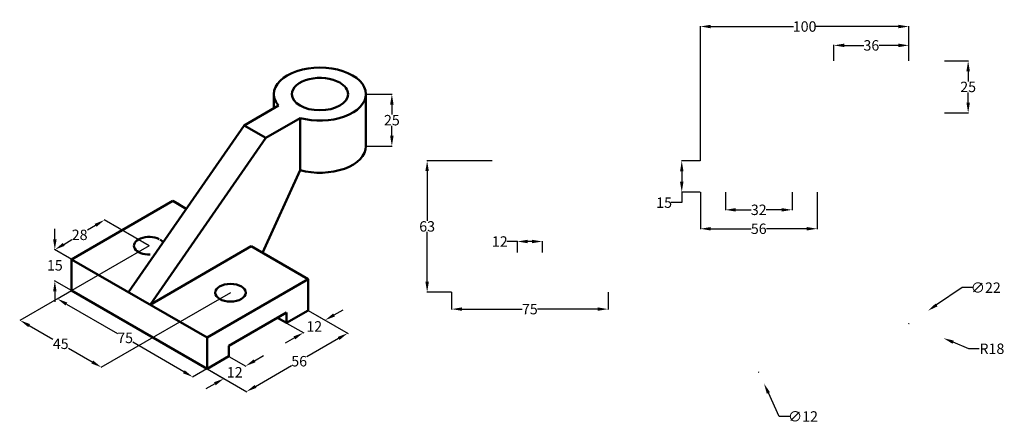
# Model space of a CAD drawing. Units: millimetres. Extents: x -452 to 20, y -1277 to -1083.
import ezdxf

# ---------------------------------------------------------------- set-up
doc = ezdxf.new("R2010")
doc.units = ezdxf.units.MM
doc.layers.add('M-DIMS', color=2, linetype='Continuous', lineweight=25)
doc.layers.add('M-OUTL', color=7, linetype='Continuous', lineweight=50)
doc.styles.get("Standard").update_dxf_attribs({"font": 'arial.ttf'})
doc.dimstyles.get("Standard").update_dxf_attribs({"dimtxt": 5, "dimasz": 5, "dimexe": 0.18, "dimexo": 0.0625, "dimgap": 0.09, "dimtad": 0, "dimtih": 1, "dimtoh": 1, "dimdec": 0, "dimzin": 0, "dimdsep": 46, "dimtxsty": 'Standard', "dimcen": 0.09, "dimadec": 0, "dimazin": 0, "dimtfac": 1, "dimtdec": 0, "dimtofl": 0, "dimtmove": 0, "dimatfit": 3, "dimfxl": 1, "dimtolj": 1, "dimtzin": 0, "dimarcsym": 0})

# ---------------------------------------------------------------- blocks, each defined once
blk = doc.blocks.new('*D1')
at = {"layer": 'Defpoints', "color": 0, "transparency": 16777216}
for p in [(-427.19, -1197.94), (-435.2, -1208.32), (-427.19, -1212.94)]:
    blk.add_point(p, dxfattribs=at)
at = {"layer": 'M-DIMS', "color": 0, "lineweight": -2, "transparency": 16777216}
for p, q in [((-435.2, -1188.32), (-435.2, -1183.32)), ((-427.25, -1197.9), (-435.38, -1193.21)), ((-427.25, -1212.9), (-435.38, -1208.21)), ((-435.2, -1213.32), (-435.2, -1218.32))]:
    blk.add_line(p, q, dxfattribs=at)
at = {"layer": 'M-DIMS', "color": 0, "transparency": 16777216}
for points in [[(-436.03, -1188.32), (-434.36, -1188.32), (-435.2, -1193.32)], [(-436.03, -1213.32), (-434.36, -1213.32), (-435.2, -1208.32)]]:
    blk.add_solid(points, dxfattribs=at)
at = {"layer": 'M-DIMS', "color": 0, "transparency": 16777216, "insert": (-435.2, -1200.82), "char_height": 5, "attachment_point": 5}
blk.add_mtext('\\A1;15', dxfattribs=at)
blk = doc.blocks.new('*D2')
at = {"layer": 'Defpoints', "color": 0, "transparency": 16777216}
for p in [(-427.19, -1212.94), (-362.24, -1250.44), (-369.03, -1254.36)]:
    blk.add_point(p, dxfattribs=at)
at = {"layer": 'M-DIMS', "color": 0, "lineweight": -2, "transparency": 16777216}
for p, q in [((-427.25, -1212.97), (-434.16, -1216.96)), ((-429.65, -1219.36), (-405.17, -1233.49)), ((-373.36, -1251.86), (-397.84, -1237.73)), ((-362.3, -1250.47), (-369.21, -1254.46))]:
    blk.add_line(p, q, dxfattribs=at)
at = {"layer": 'M-DIMS', "color": 0, "transparency": 16777216}
for points in [[(-429.23, -1218.64), (-430.07, -1220.08), (-433.98, -1216.86)], [(-372.94, -1251.14), (-373.78, -1252.58), (-369.03, -1254.36)]]:
    blk.add_solid(points, dxfattribs=at)
at = {"layer": 'M-DIMS', "color": 0, "transparency": 16777216, "insert": (-401.51, -1235.61), "char_height": 5, "attachment_point": 5}
blk.add_mtext('\\A1;75', dxfattribs=at)
blk = doc.blocks.new('*D3')
at = {"layer": 'Defpoints', "color": 0, "transparency": 16777216}
for p in [(-313.74, -1222.44), (-294.8, -1233.37), (-362.24, -1250.44)]:
    blk.add_point(p, dxfattribs=at)
at = {"layer": 'M-DIMS', "color": 0, "lineweight": -2, "transparency": 16777216}
for p, q in [((-313.68, -1222.47), (-294.62, -1233.48)), ((-299.13, -1235.87), (-314.38, -1244.68)), ((-362.17, -1250.47), (-343.12, -1261.48)), ((-338.97, -1258.87), (-321.72, -1248.91))]:
    blk.add_line(p, q, dxfattribs=at)
at = {"layer": 'M-DIMS', "color": 0, "transparency": 16777216}
for points in [[(-299.55, -1235.15), (-298.72, -1236.59), (-294.8, -1233.37)], [(-339.39, -1258.15), (-338.55, -1259.59), (-343.3, -1261.37)]]:
    blk.add_solid(points, dxfattribs=at)
at = {"layer": 'M-DIMS', "color": 0, "transparency": 16777216, "insert": (-318.05, -1246.79), "char_height": 5, "attachment_point": 5}
blk.add_mtext('\\A1;56', dxfattribs=at)
blk = doc.blocks.new('*D4')
at = {"layer": 'Defpoints', "color": 0, "transparency": 16777216}
for p in [(-313.74, -1222.44), (-305.64, -1227.11), (-324.13, -1228.44)]:
    blk.add_point(p, dxfattribs=at)
at = {"layer": 'M-DIMS', "color": 0, "lineweight": -2, "transparency": 16777216}
for p, q in [((-313.68, -1222.47), (-305.46, -1227.22)), ((-301.31, -1224.61), (-296.98, -1222.11)), ((-324.07, -1228.47), (-315.86, -1233.22)), ((-320.37, -1235.61), (-324.7, -1238.11))]:
    blk.add_line(p, q, dxfattribs=at)
at = {"layer": 'M-DIMS', "color": 0, "transparency": 16777216}
for points in [[(-301.73, -1223.89), (-300.9, -1225.33), (-305.64, -1227.11)], [(-320.78, -1234.89), (-319.95, -1236.33), (-316.04, -1233.11)]]:
    blk.add_solid(points, dxfattribs=at)
at = {"layer": 'M-DIMS', "color": 0, "transparency": 16777216, "insert": (-310.84, -1230.11), "char_height": 5, "attachment_point": 5}
blk.add_mtext('\\A1;12', dxfattribs=at)
blk = doc.blocks.new('*D5')
at = {"layer": 'Defpoints', "color": 0, "transparency": 16777216}
for p in [(-351.85, -1244.44), (-362.24, -1250.44), (-343.75, -1249.11)]:
    blk.add_point(p, dxfattribs=at)
at = {"layer": 'M-DIMS', "color": 0, "lineweight": -2, "transparency": 16777216}
for p, q in [((-351.78, -1244.47), (-343.57, -1249.22)), ((-339.42, -1246.61), (-335.09, -1244.11)), ((-362.17, -1250.47), (-353.96, -1255.22)), ((-358.47, -1257.61), (-362.8, -1260.11))]:
    blk.add_line(p, q, dxfattribs=at)
at = {"layer": 'M-DIMS', "color": 0, "transparency": 16777216}
for points in [[(-339.84, -1245.89), (-339, -1247.33), (-343.75, -1249.11)], [(-358.89, -1256.89), (-358.06, -1258.33), (-354.14, -1255.11)]]:
    blk.add_solid(points, dxfattribs=at)
at = {"layer": 'M-DIMS', "color": 0, "transparency": 16777216, "insert": (-348.95, -1252.11), "char_height": 5, "attachment_point": 5}
blk.add_mtext('\\A1;12', dxfattribs=at)
blk = doc.blocks.new('*D6')
at = {"layer": 'Defpoints', "color": 0, "transparency": 16777216}
for p in [(-435.2, -1193.32), (-389.95, -1191.44), (-413.75, -1205.7)]:
    blk.add_point(p, dxfattribs=at)
at = {"layer": 'M-DIMS', "color": 0, "lineweight": -2, "transparency": 16777216}
for p, q in [((-390.01, -1191.4), (-411.57, -1178.95)), ((-415.68, -1181.63), (-419.58, -1183.96)), ((-430.91, -1190.75), (-427.01, -1188.41)), ((-413.81, -1205.66), (-435.38, -1193.21))]:
    blk.add_line(p, q, dxfattribs=at)
at = {"layer": 'M-DIMS', "color": 0, "transparency": 16777216}
for points in [[(-416.11, -1180.91), (-415.26, -1182.34), (-411.39, -1179.06)], [(-431.34, -1190.03), (-430.48, -1191.46), (-435.2, -1193.32)]]:
    blk.add_solid(points, dxfattribs=at)
at = {"layer": 'M-DIMS', "color": 0, "transparency": 16777216, "insert": (-423.3, -1186.19), "char_height": 5, "attachment_point": 5}
blk.add_mtext('\\A1;28', dxfattribs=at)
blk = doc.blocks.new('*D7')
at = {"layer": 'Defpoints', "color": 0, "transparency": 16777216}
for p in [(-389.95, -1191.44), (-350.98, -1213.94), (-412.9, -1249.69)]:
    blk.add_point(p, dxfattribs=at)
at = {"layer": 'M-DIMS', "color": 0, "lineweight": -2, "transparency": 16777216}
for p, q in [((-390.01, -1191.47), (-452.05, -1227.29)), ((-351.04, -1213.97), (-413.08, -1249.79)), ((-447.54, -1229.69), (-436.18, -1236.25)), ((-417.23, -1247.19), (-428.6, -1240.63))]:
    blk.add_line(p, q, dxfattribs=at)
at = {"layer": 'M-DIMS', "color": 0, "transparency": 16777216}
for points in [[(-447.13, -1228.97), (-447.96, -1230.41), (-451.87, -1227.19)], [(-416.82, -1246.47), (-417.65, -1247.91), (-412.9, -1249.69)]]:
    blk.add_solid(points, dxfattribs=at)
at = {"layer": 'M-DIMS', "color": 0, "transparency": 16777216, "insert": (-432.39, -1238.44), "char_height": 5, "attachment_point": 5}
blk.add_mtext('\\A1;45', dxfattribs=at)
blk = doc.blocks.new('*D8')
at = {"layer": 'Defpoints', "color": 0, "transparency": 16777216}
for p in [(-244.95, -1213.64), (-169.95, -1213.64), (-244.95, -1221.81)]:
    blk.add_point(p, dxfattribs=at)
at = {"layer": 'M-DIMS', "color": 0, "lineweight": -2, "transparency": 16777216}
for p, q in [((-244.95, -1213.71), (-244.95, -1221.99)), ((-169.95, -1213.71), (-169.95, -1221.99)), ((-239.95, -1221.81), (-211.12, -1221.81)), ((-174.95, -1221.81), (-203.78, -1221.81))]:
    blk.add_line(p, q, dxfattribs=at)
at = {"layer": 'M-DIMS', "color": 0, "transparency": 16777216}
for points in [[(-239.95, -1220.98), (-239.95, -1222.64), (-244.95, -1221.81)], [(-174.95, -1220.98), (-174.95, -1222.64), (-169.95, -1221.81)]]:
    blk.add_solid(points, dxfattribs=at)
at = {"layer": 'M-DIMS', "color": 0, "transparency": 16777216, "insert": (-207.45, -1221.81), "char_height": 5, "attachment_point": 5}
blk.add_mtext('\\A1;75', dxfattribs=at)
blk = doc.blocks.new('*D9')
at = {"layer": 'Defpoints', "color": 0, "transparency": 16777216}
for p in [(-125.71, -1150.74), (-134.62, -1165.74), (-125.71, -1165.74)]:
    blk.add_point(p, dxfattribs=at)
at = {"layer": 'M-DIMS', "color": 0, "lineweight": -2, "transparency": 16777216}
for p, q in [((-125.78, -1150.74), (-134.8, -1150.74)), ((-134.62, -1155.74), (-134.62, -1160.74)), ((-125.78, -1165.74), (-134.8, -1165.74)), ((-134.62, -1165.74), (-134.62, -1170.74)), ((-134.62, -1170.74), (-139.62, -1170.74))]:
    blk.add_line(p, q, dxfattribs=at)
at = {"layer": 'M-DIMS', "color": 0, "transparency": 16777216}
for points in [[(-135.45, -1155.74), (-133.78, -1155.74), (-134.62, -1150.74)], [(-135.45, -1160.74), (-133.78, -1160.74), (-134.62, -1165.74)]]:
    blk.add_solid(points, dxfattribs=at)
at = {"layer": 'M-DIMS', "color": 0, "transparency": 16777216, "insert": (-143.07, -1170.74), "char_height": 5, "attachment_point": 5}
blk.add_mtext('\\A1;15', dxfattribs=at)
blk = doc.blocks.new('*D10')
at = {"layer": 'Defpoints', "color": 0, "transparency": 16777216}
for p in [(-113.71, -1165.74), (-81.71, -1165.74), (-81.71, -1174.19)]:
    blk.add_point(p, dxfattribs=at)
at = {"layer": 'M-DIMS', "color": 0, "lineweight": -2, "transparency": 16777216}
for p, q in [((-113.71, -1165.8), (-113.71, -1174.37)), ((-81.71, -1165.8), (-81.71, -1174.37)), ((-108.71, -1174.19), (-101.36, -1174.19)), ((-86.71, -1174.19), (-94.07, -1174.19))]:
    blk.add_line(p, q, dxfattribs=at)
at = {"layer": 'M-DIMS', "color": 0, "transparency": 16777216}
for points in [[(-108.71, -1173.36), (-108.71, -1175.02), (-113.71, -1174.19)], [(-86.71, -1173.36), (-86.71, -1175.02), (-81.71, -1174.19)]]:
    blk.add_solid(points, dxfattribs=at)
at = {"layer": 'M-DIMS', "color": 0, "transparency": 16777216, "insert": (-97.71, -1174.19), "char_height": 5, "attachment_point": 5}
blk.add_mtext('\\A1;32', dxfattribs=at)
blk = doc.blocks.new('*D11')
at = {"layer": 'Defpoints', "color": 0, "transparency": 16777216}
for p in [(-125.71, -1165.74), (-69.71, -1165.74), (-69.71, -1183.27)]:
    blk.add_point(p, dxfattribs=at)
at = {"layer": 'M-DIMS', "color": 0, "lineweight": -2, "transparency": 16777216}
for p, q in [((-125.71, -1165.8), (-125.71, -1183.45)), ((-69.71, -1165.8), (-69.71, -1183.45)), ((-120.71, -1183.27), (-101.38, -1183.27)), ((-74.71, -1183.27), (-94.04, -1183.27))]:
    blk.add_line(p, q, dxfattribs=at)
at = {"layer": 'M-DIMS', "color": 0, "transparency": 16777216}
for points in [[(-120.71, -1182.44), (-120.71, -1184.11), (-125.71, -1183.27)], [(-74.71, -1182.44), (-74.71, -1184.11), (-69.71, -1183.27)]]:
    blk.add_solid(points, dxfattribs=at)
at = {"layer": 'M-DIMS', "color": 0, "transparency": 16777216, "insert": (-97.71, -1183.27), "char_height": 5, "attachment_point": 5}
blk.add_mtext('\\A1;56', dxfattribs=at)
blk = doc.blocks.new('*D12')
at = {"layer": 'Defpoints', "color": 0, "transparency": 16777216}
for p in [(-8.71, -1102.74), (2.7, -1102.74), (-8.71, -1127.74)]:
    blk.add_point(p, dxfattribs=at)
at = {"layer": 'M-DIMS', "color": 0, "lineweight": -2, "transparency": 16777216}
for p, q in [((-8.65, -1102.74), (2.88, -1102.74)), ((2.7, -1107.74), (2.7, -1112.6)), ((2.7, -1122.74), (2.7, -1117.88)), ((-8.65, -1127.74), (2.88, -1127.74))]:
    blk.add_line(p, q, dxfattribs=at)
at = {"layer": 'M-DIMS', "color": 0, "transparency": 16777216}
for points in [[(1.86, -1107.74), (3.53, -1107.74), (2.7, -1102.74)], [(1.86, -1122.74), (3.53, -1122.74), (2.7, -1127.74)]]:
    blk.add_solid(points, dxfattribs=at)
at = {"layer": 'M-DIMS', "color": 0, "transparency": 16777216, "insert": (2.7, -1115.24), "char_height": 5, "attachment_point": 5}
blk.add_mtext('\\A1;25', dxfattribs=at)
blk = doc.blocks.new('*D13')
at = {"layer": 'Defpoints', "color": 0, "transparency": 16777216}
for p in [(-25.71, -1095.32), (-61.71, -1102.74), (-25.71, -1102.74)]:
    blk.add_point(p, dxfattribs=at)
at = {"layer": 'M-DIMS', "color": 0, "lineweight": -2, "transparency": 16777216}
for p, q in [((-61.71, -1102.68), (-61.71, -1095.14)), ((-25.71, -1102.68), (-25.71, -1095.14)), ((-56.71, -1095.32), (-47.38, -1095.32)), ((-30.71, -1095.32), (-40.05, -1095.32))]:
    blk.add_line(p, q, dxfattribs=at)
at = {"layer": 'M-DIMS', "color": 0, "transparency": 16777216}
for points in [[(-56.71, -1094.49), (-56.71, -1096.16), (-61.71, -1095.32)], [(-30.71, -1094.49), (-30.71, -1096.16), (-25.71, -1095.32)]]:
    blk.add_solid(points, dxfattribs=at)
at = {"layer": 'M-DIMS', "color": 0, "transparency": 16777216, "insert": (-43.71, -1095.32), "char_height": 5, "attachment_point": 5}
blk.add_mtext('\\A1;36', dxfattribs=at)
blk = doc.blocks.new('*D14')
at = {"layer": 'Defpoints', "color": 0, "transparency": 16777216}
for p in [(-125.71, -1086.28), (-25.71, -1102.74), (-125.71, -1150.74)]:
    blk.add_point(p, dxfattribs=at)
at = {"layer": 'M-DIMS', "color": 0, "lineweight": -2, "transparency": 16777216}
for p, q in [((-125.71, -1150.68), (-125.71, -1086.1)), ((-120.71, -1086.28), (-81.08, -1086.28)), ((-30.71, -1086.28), (-70.34, -1086.28)), ((-25.71, -1102.68), (-25.71, -1086.1))]:
    blk.add_line(p, q, dxfattribs=at)
at = {"layer": 'M-DIMS', "color": 0, "transparency": 16777216}
for points in [[(-120.71, -1085.45), (-120.71, -1087.12), (-125.71, -1086.28)], [(-30.71, -1085.45), (-30.71, -1087.12), (-25.71, -1086.28)]]:
    blk.add_solid(points, dxfattribs=at)
at = {"layer": 'M-DIMS', "color": 0, "transparency": 16777216, "insert": (-75.71, -1086.28), "char_height": 5, "attachment_point": 5}
blk.add_mtext('\\A1;100', dxfattribs=at)
blk = doc.blocks.new('*D15')
at = {"layer": 'Defpoints', "color": 0, "transparency": 16777216}
for p in [(-16.6, -1222.61), (-34.82, -1234.95)]:
    blk.add_point(p, dxfattribs=at)
at = {"layer": 'M-DIMS', "color": 0, "lineweight": -2, "transparency": 16777216}
for p, q in [((-0.23, -1211.52), (-12.46, -1219.81)), ((4.77, -1211.52), (-0.23, -1211.52)), ((-25.8, -1228.78), (-25.62, -1228.78)), ((-25.71, -1228.87), (-25.71, -1228.69))]:
    blk.add_line(p, q, dxfattribs=at)
at = {"layer": 'M-DIMS', "color": 0, "transparency": 16777216}
blk.add_solid([(-12.93, -1219.12), (-12, -1220.5), (-16.6, -1222.61)], dxfattribs=at)
at = {"layer": 'M-DIMS', "color": 0, "transparency": 16777216, "insert": (11.14, -1211.52), "char_height": 5, "attachment_point": 5}
blk.add_mtext('\\A1;∅22', dxfattribs=at)
blk = doc.blocks.new('*D16')
at = {"layer": 'Defpoints', "color": 0, "transparency": 16777216}
for p in [(-25.71, -1228.78), (-9.11, -1235.73)]:
    blk.add_point(p, dxfattribs=at)
at = {"layer": 'M-DIMS', "color": 0, "lineweight": -2, "transparency": 16777216}
for p, q in [((-25.8, -1228.78), (-25.62, -1228.78)), ((-25.71, -1228.87), (-25.71, -1228.69)), ((3.01, -1240.81), (-4.5, -1237.66)), ((8.01, -1240.81), (3.01, -1240.81))]:
    blk.add_line(p, q, dxfattribs=at)
at = {"layer": 'M-DIMS', "color": 0, "transparency": 16777216}
blk.add_solid([(-4.18, -1236.9), (-4.82, -1238.43), (-9.11, -1235.73)], dxfattribs=at)
at = {"layer": 'M-DIMS', "color": 0, "transparency": 16777216, "insert": (14.08, -1240.81), "char_height": 5, "attachment_point": 5}
blk.add_mtext('\\A1;R18', dxfattribs=at)
blk = doc.blocks.new('*D17')
at = {"layer": 'Defpoints', "color": 0, "transparency": 16777216}
for p in [(-100.23, -1246.59), (-95.19, -1257.48)]:
    blk.add_point(p, dxfattribs=at)
at = {"layer": 'M-DIMS', "color": 0, "lineweight": -2, "transparency": 16777216}
for p, q in [((-97.8, -1252.03), (-97.62, -1252.03)), ((-97.71, -1252.12), (-97.71, -1251.94)), ((-87.87, -1273.29), (-93.09, -1262.01)), ((-82.87, -1273.29), (-87.87, -1273.29))]:
    blk.add_line(p, q, dxfattribs=at)
at = {"layer": 'M-DIMS', "color": 0, "transparency": 16777216}
blk.add_solid([(-92.34, -1261.66), (-93.85, -1262.36), (-95.19, -1257.48)], dxfattribs=at)
at = {"layer": 'M-DIMS', "color": 0, "transparency": 16777216, "insert": (-76.5, -1273.29), "char_height": 5, "attachment_point": 5}
blk.add_mtext('\\A1;∅12', dxfattribs=at)
blk = doc.blocks.new('*D18')
at = {"layer": 'Defpoints', "color": 0, "transparency": 16777216}
for p in [(-256.7, -1150.64), (-225.45, -1150.64), (-244.95, -1213.64)]:
    blk.add_point(p, dxfattribs=at)
at = {"layer": 'M-DIMS', "color": 0, "lineweight": -2, "transparency": 16777216}
for p, q in [((-225.51, -1150.64), (-256.88, -1150.64)), ((-256.7, -1155.64), (-256.7, -1179.5)), ((-256.7, -1208.64), (-256.7, -1184.79)), ((-245.01, -1213.64), (-256.88, -1213.64))]:
    blk.add_line(p, q, dxfattribs=at)
at = {"layer": 'M-DIMS', "color": 0, "transparency": 16777216}
for points in [[(-257.54, -1155.64), (-255.87, -1155.64), (-256.7, -1150.64)], [(-257.54, -1208.64), (-255.87, -1208.64), (-256.7, -1213.64)]]:
    blk.add_solid(points, dxfattribs=at)
at = {"layer": 'M-DIMS', "color": 0, "transparency": 16777216, "insert": (-256.7, -1182.14), "char_height": 5, "attachment_point": 5}
blk.add_mtext('\\A1;63', dxfattribs=at)
blk = doc.blocks.new('*D19')
at = {"layer": 'Defpoints', "color": 0, "transparency": 16777216}
for p in [(-213.45, -1189.38), (-213.45, -1194.64), (-201.45, -1194.64)]:
    blk.add_point(p, dxfattribs=at)
at = {"layer": 'M-DIMS', "color": 0, "lineweight": -2, "transparency": 16777216}
for p, q in [((-213.45, -1189.38), (-218.45, -1189.38)), ((-213.45, -1194.58), (-213.45, -1189.2)), ((-206.45, -1189.38), (-208.45, -1189.38)), ((-201.45, -1194.58), (-201.45, -1189.2))]:
    blk.add_line(p, q, dxfattribs=at)
at = {"layer": 'M-DIMS', "color": 0, "transparency": 16777216}
for points in [[(-208.45, -1188.55), (-208.45, -1190.22), (-213.45, -1189.38)], [(-206.45, -1188.55), (-206.45, -1190.22), (-201.45, -1189.38)]]:
    blk.add_solid(points, dxfattribs=at)
at = {"layer": 'M-DIMS', "color": 0, "transparency": 16777216, "insert": (-221.86, -1189.38), "char_height": 5, "attachment_point": 5}
blk.add_mtext('\\A1;12', dxfattribs=at)
blk = doc.blocks.new('*D20')
at = {"layer": 'Defpoints', "color": 0, "transparency": 16777216}
for p in [(-286.07, -1118.69), (-286.07, -1143.69), (-273.61, -1143.69)]:
    blk.add_point(p, dxfattribs=at)
at = {"layer": 'M-DIMS', "color": 0, "lineweight": -2, "transparency": 16777216}
for p, q in [((-286, -1118.69), (-273.43, -1118.69)), ((-273.61, -1123.69), (-273.61, -1128.55)), ((-273.61, -1138.69), (-273.61, -1133.83)), ((-286, -1143.69), (-273.43, -1143.69))]:
    blk.add_line(p, q, dxfattribs=at)
at = {"layer": 'M-DIMS', "color": 0, "transparency": 16777216}
for points in [[(-274.44, -1123.69), (-272.78, -1123.69), (-273.61, -1118.69)], [(-274.44, -1138.69), (-272.78, -1138.69), (-273.61, -1143.69)]]:
    blk.add_solid(points, dxfattribs=at)
at = {"layer": 'M-DIMS', "color": 0, "transparency": 16777216, "insert": (-273.61, -1131.19), "char_height": 5, "attachment_point": 5}
blk.add_mtext('\\A1;25', dxfattribs=at)

msp = doc.modelspace()

# ---------------------------------------------------------------- linework, layer by layer
at = {"layer": 'M-OUTL'}
for p, q in [((-330.16, -1125.42), (-330.16, -1118.69)), ((-286.07, -1143.69), (-286.07, -1118.69)), ((-344.48, -1133.69), (-328, -1124.17)), ((-334.09, -1139.69), (-317.61, -1130.17)), ((-317.61, -1155.17), (-317.61, -1130.17)), ((-399.91, -1213.69), (-344.48, -1133.69)), ((-334.09, -1139.69), (-344.48, -1133.69)), ((-389.52, -1219.69), (-334.09, -1139.69)), ((-317.61, -1155.17), (-335.62, -1194.81)), ((-427.19, -1197.94), (-378.69, -1169.94)), ((-378.69, -1169.94), (-375.66, -1171.69)), ((-372.2, -1173.69), (-378.69, -1169.94)), ((-389.52, -1219.69), (-341.02, -1191.69)), ((-341.02, -1191.69), (-313.74, -1207.44)), ((-362.24, -1235.44), (-427.19, -1197.94)), ((-427.19, -1197.94), (-427.19, -1212.94)), ((-362.24, -1235.44), (-313.74, -1207.44)), ((-313.74, -1207.44), (-313.74, -1222.44)), ((-427.19, -1212.94), (-362.24, -1250.44)), ((-313.74, -1222.44), (-324.13, -1228.44)), ((-351.85, -1239.44), (-324.13, -1223.44)), ((-324.13, -1228.44), (-328.46, -1225.94)), ((-324.13, -1228.44), (-324.13, -1223.44)), ((-362.24, -1250.44), (-362.24, -1235.44)), ((-351.85, -1244.44), (-351.85, -1239.44)), ((-362.24, -1250.44), (-351.85, -1244.44))]:
    msp.add_line(p, q, dxfattribs=at)
for centre, major_axis, start_param, end_param in [((-308.11, -1118.69), (22.05, 0), 0, 3.141593), ((-308.11, -1118.69), (13.47, 0), 0.785398, 3.141593), ((-308.11, -1118.69), (13.47, 0), 0, 0.785398), ((-308.11, -1118.69), (22.05, 0), 3.141593, 3.587154), ((-308.11, -1118.69), (13.47, 0), 3.141593, 6.283185), ((-308.11, -1118.69), (22.05, 0), 4.266828, 6.283185), ((-308.11, -1143.69), (22.05, 0), 4.266828, 6.283185), ((-389.95, -1191.44), (-7.35, 0), 4.008745, 7.914124), ((-389.95, -1191.44), (7.35, 0), 0.429686, 0.785398)]:
    msp.add_ellipse(centre, major_axis=major_axis, ratio=0.57735, start_param=start_param, end_param=end_param, dxfattribs=at)
msp.add_ellipse((-350.98, -1213.94), major_axis=(-7.35, 0), ratio=0.57735, dxfattribs=at)

# ---------------------------------------------------------------- dimensions: what is measured, and where the dimension line sits
at = {"layer": 'M-DIMS'}
for base, p1, p2, picture, middle in [((-125.71, -1086.28), (-25.71, -1102.74), (-125.71, -1150.74), '*D14', (-75.71, -1086.28)), ((-25.71, -1095.32), (-61.71, -1102.74), (-25.71, -1102.74), '*D13', (-43.71, -1095.32)), ((-69.71, -1183.27), (-125.71, -1165.74), (-69.71, -1165.74), '*D11', (-97.71, -1183.27)), ((-81.71, -1174.19), (-113.71, -1165.74), (-81.71, -1165.74), '*D10', (-97.71, -1174.19)), ((-213.45, -1189.38), (-201.45, -1194.64), (-213.45, -1194.64), '*D19', (-221.86, -1189.38)), ((-244.95, -1221.81), (-169.95, -1213.64), (-244.95, -1213.64), '*D8', (-207.45, -1221.81))]:
    dim = msp.add_linear_dim(base=base, p1=p1, p2=p2, dimstyle='Standard', override={"dimclrd": 0, "dimclre": 0, "dimclrt": 0}, dxfattribs=at)
    dim.commit()
    dim.dimension.update_dxf_attribs({"geometry": picture, "text_midpoint": middle})
for base, p1, p2, angle, override, picture, middle in [((2.7, -1102.74), (-8.71, -1127.74), (-8.71, -1102.74), 90, {"dimclrd": 0, "dimclre": 0, "dimclrt": 0}, '*D12', (2.7, -1115.24)), ((-273.61, -1143.69), (-286.07, -1118.69), (-286.07, -1143.69), 270, {"dimrnd": 0}, '*D20', (-273.61, -1131.19)), ((-256.7, -1150.64), (-244.95, -1213.64), (-225.45, -1150.64), 90, {"dimclrd": 0, "dimclre": 0, "dimclrt": 0}, '*D18', (-256.7, -1182.14)), ((-134.62, -1165.74), (-125.71, -1150.74), (-125.71, -1165.74), 90, {"dimclrd": 0, "dimclre": 0, "dimclrt": 0}, '*D9', (-143.07, -1170.74))]:
    dim = msp.add_linear_dim(base=base, p1=p1, p2=p2, angle=angle, dimstyle='Standard', override=override, dxfattribs=at)
    dim.commit()
    dim.dimension.update_dxf_attribs({"geometry": picture, "text_midpoint": middle})
for p1, p2, distance, picture, middle in [((-389.95, -1191.44), (-413.75, -1205.7), -21.64, '*D6', (-423.3, -1186.19)), ((-389.95, -1191.44), (-350.98, -1213.94), -61.92, '*D7', (-432.39, -1238.44)), ((-427.19, -1212.94), (-362.24, -1250.44), -6.79, '*D2', (-401.51, -1235.61))]:
    dim = msp.add_aligned_dim(p1=p1, p2=p2, distance=distance, dimstyle='Standard', override={"dimclrd": 0, "dimclre": 0, "dimclrt": 0}, dxfattribs=at)
    dim.commit()
    dim.dimension.update_dxf_attribs({"geometry": picture, "text_midpoint": middle})
for base, p1, p2, angle, picture, middle, dimtype in [((-435.2, -1208.32), (-427.19, -1197.94), (-427.19, -1212.94), 90, '*D1', (-435.2, -1200.82), 160), ((-294.8, -1233.37), (-362.24, -1250.44), (-313.74, -1222.44), 30, '*D3', (-318.05, -1246.79), 161), ((-305.64, -1227.11), (-324.13, -1228.44), (-313.74, -1222.44), 30, '*D4', (-310.84, -1230.11), 161), ((-343.75, -1249.11), (-362.24, -1250.44), (-351.85, -1244.44), 30, '*D5', (-348.95, -1252.11), 161)]:
    dim = msp.add_linear_dim(base=base, p1=p1, p2=p2, angle=angle, dimstyle='Standard', override={"dimclrd": 0, "dimclre": 0, "dimclrt": 0}, dxfattribs=at)
    dim.commit()
    dim.dimension.update_dxf_attribs({"geometry": picture, "text_midpoint": middle, "dimtype": dimtype})
for p1, p2, picture, middle in [((-34.82, -1234.95), (-16.6, -1222.61), '*D15', (11.14, -1211.52)), ((-100.23, -1246.59), (-95.19, -1257.48), '*D17', (-76.5, -1273.29))]:
    dim = msp.add_diameter_dim_2p(p1=p1, p2=p2, dimstyle='Standard', override={"dimclrd": 0, "dimclre": 0, "dimclrt": 0}, dxfattribs=at)
    dim.commit()
    dim.dimension.update_dxf_attribs({"geometry": picture, "text_midpoint": middle, "dimtype": 163})
dim = msp.add_radius_dim(center=(-25.71, -1228.78), mpoint=(-9.11, -1235.73), dimstyle='Standard', override={"dimclrd": 0, "dimclre": 0, "dimclrt": 0}, dxfattribs=at)
dim.commit()
dim.dimension.update_dxf_attribs({"geometry": '*D16', "text_midpoint": (14.08, -1240.81), "dimtype": 164})

doc.saveas('drawing.dxf')
